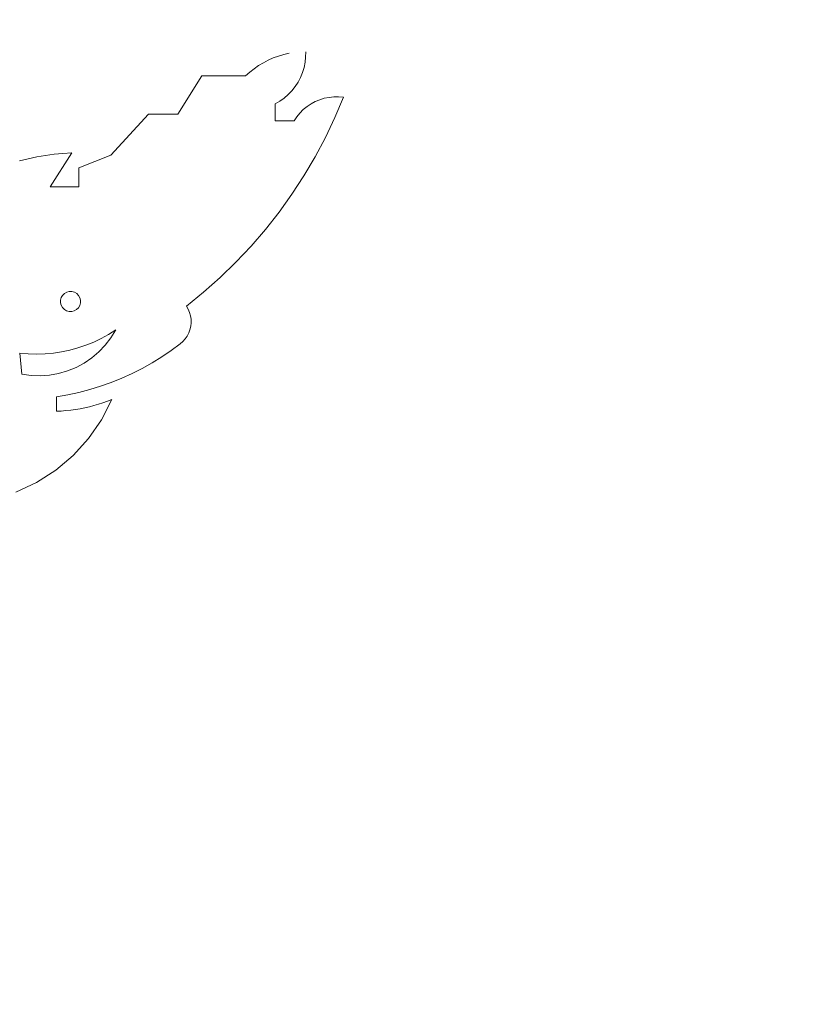
# Model space of a CAD drawing. Units: millimetres. Extents: x 7894 to 8038, y 6851 to 6951.
# Tile 31 of 49: x 7960.68 to 7962.874, y 6925.713 to 6928.453. Entities that reach past the tile are written whole.
import ezdxf

# ---------------------------------------------------------------- set-up
doc = ezdxf.new("R2010")
doc.units = ezdxf.units.MM
doc.layers.add('A-ANNO-DIMS', color=2, linetype='Continuous', lineweight=18)
doc.layers.add('A-FURN-ACCS', color=8, linetype='Continuous', lineweight=13)
doc.styles.get("Standard").update_dxf_attribs({"font": 'arial.ttf'})
doc.dimstyles.new('ISO-25', dxfattribs={"dimtxt": 1, "dimasz": 1, "dimexe": 1.25, "dimexo": 0.625, "dimtad": 1, "dimdec": 0, "dimlunit": 4, "dimtxsty": 'Standard', "dimcen": 2.5, "dimclrt": 1, "dimadec": 0, "dimazin": 0, "dimtfac": 1, "dimtdec": 0, "dimtmove": 0, "dimatfit": 3, "dimfxl": 1, "dimarcsym": 0})

# ---------------------------------------------------------------- blocks, each defined once
blk = doc.blocks.new('DISPLAY-LEAF-FINIAL-Z2_152')
for p, q in [((2.565, 3.5085, 2.1518), (2.5649, 3.4937, 2.1518)), ((2.4472, 3.4779, 2.1518), (2.4609, 3.4849, 2.1518)), ((2.4609, 3.4849, 2.1518), (2.4749, 3.4911, 2.1518)), ((2.4749, 3.4911, 2.1518), (2.4894, 3.4964, 2.1518)), ((2.4894, 3.4964, 2.1518), (2.5041, 3.5007, 2.1518)), ((2.5041, 3.5007, 2.1518), (2.5191, 3.5041, 2.1518)), ((2.5649, 3.4937, 2.1518), (2.5634, 3.479, 2.1518)), ((2.4094, 3.4516, 2.1518), (2.4214, 3.4612, 2.1518)), ((2.4214, 3.4612, 2.1518), (2.4341, 3.4699, 2.1518)), ((2.4341, 3.4699, 2.1518), (2.4472, 3.4779, 2.1518)), ((2.5605, 3.4646, 2.1518), (2.5562, 3.4504, 2.1518)), ((2.5634, 3.479, 2.1518), (2.5605, 3.4646, 2.1518)), ((2.2094, 3.3343, 2.1518), (2.2756, 3.4413, 2.1518)), ((2.2756, 3.4413, 2.1518), (2.3979, 3.4413, 2.1518)), ((2.3979, 3.4413, 2.1518), (2.4094, 3.4516, 2.1518)), ((2.5507, 3.4368, 2.1518), (2.5438, 3.4237, 2.1518)), ((2.5562, 3.4504, 2.1518), (2.5507, 3.4368, 2.1518)), ((2.5266, 3.3997, 2.1518), (2.5164, 3.3891, 2.1518)), ((2.5358, 3.4113, 2.1518), (2.5266, 3.3997, 2.1518)), ((2.5438, 3.4237, 2.1518), (2.5358, 3.4113, 2.1518)), ((2.4932, 3.3709, 2.1518), (2.4804, 3.3636, 2.1518)), ((2.5052, 3.3794, 2.1518), (2.4932, 3.3709, 2.1518)), ((2.5164, 3.3891, 2.1518), (2.5052, 3.3794, 2.1518)), ((2.5917, 3.3696, 2.1518), (2.604, 3.3748, 2.1518)), ((2.604, 3.3748, 2.1518), (2.6168, 3.3788, 2.1518)), ((2.6168, 3.3788, 2.1518), (2.63, 3.3815, 2.1518)), ((2.63, 3.3815, 2.1518), (2.6433, 3.3829, 2.1518)), ((2.6433, 3.3829, 2.1518), (2.6567, 3.3831, 2.1518)), ((2.6701, 3.3819, 2.1518), (2.6462, 3.3254, 2.1518)), ((2.6567, 3.3831, 2.1518), (2.6701, 3.3819, 2.1518)), ((2.4804, 3.3636, 2.1518), (2.4804, 3.3164, 2.1518)), ((2.5489, 3.3378, 2.1518), (2.5584, 3.3473, 2.1518)), ((2.5584, 3.3473, 2.1518), (2.5687, 3.3558, 2.1518)), ((2.5687, 3.3558, 2.1518), (2.5799, 3.3633, 2.1518)), ((2.5799, 3.3633, 2.1518), (2.5917, 3.3696, 2.1518)), ((2.0233, 3.2209, 2.1518), (2.1272, 3.3343, 2.1518)), ((2.1272, 3.3343, 2.1518), (2.2094, 3.3343, 2.1518)), ((2.4804, 3.3164, 2.1518), (2.5329, 3.3164, 2.1518)), ((2.5329, 3.3164, 2.1518), (2.5403, 3.3275, 2.1518)), ((2.5403, 3.3275, 2.1518), (2.5489, 3.3378, 2.1518)), ((2.6462, 3.3254, 2.1518), (2.6199, 3.27, 2.1518)), ((2.6199, 3.27, 2.1518), (2.5912, 3.2159, 2.1518)), ((1.7688, 3.2049, 2.1518), (1.7926, 3.2108, 2.1518)), ((1.7926, 3.2108, 2.1518), (1.8166, 3.2158, 2.1518)), ((1.8166, 3.2158, 2.1518), (1.8408, 3.2199, 2.1518)), ((1.8408, 3.2199, 2.1518), (1.8651, 3.2232, 2.1518)), ((1.9139, 3.2271, 2.1518), (1.8536, 3.1329, 2.1518)), ((1.8651, 3.2232, 2.1518), (1.8895, 3.2256, 2.1518)), ((1.8895, 3.2256, 2.1518), (1.9139, 3.2271, 2.1518)), ((1.934, 3.1854, 2.1518), (2.0233, 3.2209, 2.1518)), ((2.5912, 3.2159, 2.1518), (2.56, 3.1631, 2.1518)), ((1.934, 3.1329, 2.1518), (1.934, 3.1854, 2.1518)), ((2.56, 3.1631, 2.1518), (2.5265, 3.1117, 2.1518)), ((1.8536, 3.1329, 2.1518), (1.934, 3.1329, 2.1518)), ((2.5265, 3.1117, 2.1518), (2.4908, 3.0619, 2.1518)), ((2.4908, 3.0619, 2.1518), (2.4529, 3.0137, 2.1518)), ((2.4529, 3.0137, 2.1518), (2.4129, 2.9672, 2.1518)), ((2.4129, 2.9672, 2.1518), (2.3708, 2.9226, 2.1518)), ((2.3708, 2.9226, 2.1518), (2.3268, 2.8799, 2.1518)), ((2.3268, 2.8799, 2.1518), (2.2809, 2.8392, 2.1518)), ((1.8829, 2.8172, 2.1518), (1.8849, 2.8243, 2.1518)), ((1.8849, 2.8243, 2.1518), (1.8885, 2.8306, 2.1518)), ((1.8885, 2.8306, 2.1518), (1.8937, 2.8357, 2.1518)), ((1.8937, 2.8357, 2.1518), (1.9001, 2.8393, 2.1518)), ((1.9001, 2.8393, 2.1518), (1.9071, 2.8412, 2.1518)), ((1.9071, 2.8412, 2.1518), (1.9144, 2.8411, 2.1518)), ((1.9144, 2.8411, 2.1518), (1.9215, 2.8392, 2.1518)), ((1.9215, 2.8392, 2.1518), (1.9278, 2.8355, 2.1518)), ((1.9278, 2.8355, 2.1518), (1.9329, 2.8304, 2.1518)), ((1.9329, 2.8304, 2.1518), (1.9365, 2.824, 2.1518)), ((1.9365, 2.824, 2.1518), (1.9384, 2.817, 2.1518)), ((2.2809, 2.8392, 2.1518), (2.2333, 2.8006, 2.1518)), ((1.8829, 2.8099, 2.1518), (1.8829, 2.8172, 2.1518)), ((1.8847, 2.8029, 2.1518), (1.8829, 2.8099, 2.1518)), ((1.8884, 2.7965, 2.1518), (1.8847, 2.8029, 2.1518)), ((1.8935, 2.7913, 2.1518), (1.8884, 2.7965, 2.1518)), ((1.9327, 2.7963, 2.1518), (1.9275, 2.7912, 2.1518)), ((1.9364, 2.8026, 2.1518), (1.9327, 2.7963, 2.1518)), ((1.9383, 2.8097, 2.1518), (1.9364, 2.8026, 2.1518)), ((1.9384, 2.817, 2.1518), (1.9383, 2.8097, 2.1518)), ((2.2333, 2.8006, 2.1518), (2.2382, 2.7921, 2.1518)), ((1.8998, 2.7877, 2.1518), (1.8935, 2.7913, 2.1518)), ((1.9068, 2.7857, 2.1518), (1.8998, 2.7877, 2.1518)), ((1.9141, 2.7857, 2.1518), (1.9068, 2.7857, 2.1518)), ((1.9212, 2.7876, 2.1518), (1.9141, 2.7857, 2.1518)), ((1.9275, 2.7912, 2.1518), (1.9212, 2.7876, 2.1518)), ((2.2382, 2.7921, 2.1518), (2.242, 2.7831, 2.1518)), ((2.242, 2.7831, 2.1518), (2.2446, 2.7737, 2.1518)), ((2.2446, 2.7737, 2.1518), (2.246, 2.7641, 2.1518)), ((2.2452, 2.7446, 2.1518), (2.243, 2.7351, 2.1518)), ((2.2462, 2.7543, 2.1518), (2.2452, 2.7446, 2.1518)), ((2.246, 2.7641, 2.1518), (2.2462, 2.7543, 2.1518)), ((2.0167, 2.7218, 2.1518), (1.9962, 2.7106, 2.1518)), ((2.023, 2.7124, 2.1518), (2.0073, 2.692, 2.1518)), ((2.0364, 2.7343, 2.1518), (2.0167, 2.7218, 2.1518)), ((2.0364, 2.7343, 2.1518), (2.023, 2.7124, 2.1518)), ((2.2352, 2.7172, 2.1518), (2.2296, 2.7092, 2.1518)), ((2.2396, 2.7259, 2.1518), (2.2352, 2.7172, 2.1518)), ((2.243, 2.7351, 2.1518), (2.2396, 2.7259, 2.1518)), ((1.9535, 2.6918, 2.1518), (1.9314, 2.6843, 2.1518)), ((1.9751, 2.7005, 2.1518), (1.9535, 2.6918, 2.1518)), ((1.9962, 2.7106, 2.1518), (1.9751, 2.7005, 2.1518)), ((2.0073, 2.692, 2.1518), (1.9895, 2.6734, 2.1518)), ((2.2158, 2.6954, 2.1518), (2.1904, 2.6768, 2.1518)), ((2.2231, 2.7019, 2.1518), (2.2158, 2.6954, 2.1518)), ((2.2296, 2.7092, 2.1518), (2.2231, 2.7019, 2.1518)), ((1.793, 2.6675, 2.1518), (1.7698, 2.6695, 2.1518)), ((1.7698, 2.6695, 2.1518), (1.7755, 2.6114, 2.1518)), ((1.8164, 2.6669, 2.1518), (1.793, 2.6675, 2.1518)), ((1.8397, 2.6677, 2.1518), (1.8164, 2.6669, 2.1518)), ((1.8629, 2.6698, 2.1518), (1.8397, 2.6677, 2.1518)), ((1.886, 2.6733, 2.1518), (1.8629, 2.6698, 2.1518)), ((1.9089, 2.6781, 2.1518), (1.886, 2.6733, 2.1518)), ((1.9314, 2.6843, 2.1518), (1.9089, 2.6781, 2.1518)), ((1.9895, 2.6734, 2.1518), (1.9699, 2.6568, 2.1518)), ((2.1643, 2.6592, 2.1518), (2.1374, 2.6427, 2.1518)), ((2.1904, 2.6768, 2.1518), (2.1643, 2.6592, 2.1518)), ((1.9261, 2.6302, 2.1518), (1.9023, 2.6205, 2.1518)), ((1.9487, 2.6423, 2.1518), (1.9261, 2.6302, 2.1518)), ((1.9699, 2.6568, 2.1518), (1.9487, 2.6423, 2.1518)), ((2.1374, 2.6427, 2.1518), (2.1099, 2.6273, 2.1518)), ((1.8009, 2.6079, 2.1518), (1.7755, 2.6114, 2.1518)), ((1.8266, 2.607, 2.1518), (1.8009, 2.6079, 2.1518)), ((1.8523, 2.6088, 2.1518), (1.8266, 2.607, 2.1518)), ((1.8776, 2.6133, 2.1518), (1.8523, 2.6088, 2.1518)), ((1.9023, 2.6205, 2.1518), (1.8776, 2.6133, 2.1518)), ((2.0818, 2.6132, 2.1518), (2.0531, 2.6002, 2.1518)), ((2.1099, 2.6273, 2.1518), (2.0818, 2.6132, 2.1518)), ((1.9942, 2.5779, 2.1518), (1.9641, 2.5686, 2.1518)), ((2.0239, 2.5884, 2.1518), (1.9942, 2.5779, 2.1518)), ((2.0531, 2.6002, 2.1518), (2.0239, 2.5884, 2.1518)), ((1.9029, 2.5539, 2.1518), (1.8718, 2.5484, 2.1518)), ((1.8718, 2.5484, 2.1518), (1.8718, 2.5082, 2.1518)), ((1.9336, 2.5606, 2.1518), (1.9029, 2.5539, 2.1518)), ((1.9641, 2.5686, 2.1518), (1.9336, 2.5606, 2.1518)), ((1.9502, 2.5177, 2.1518), (1.9631, 2.5206, 2.1518)), ((1.9631, 2.5206, 2.1518), (1.9758, 2.5239, 2.1518)), ((1.9758, 2.5239, 2.1518), (1.9885, 2.5276, 2.1518)), ((1.9885, 2.5276, 2.1518), (2.001, 2.5317, 2.1518)), ((2.0257, 2.5409, 2.1518), (1.9968, 2.4843, 2.1518)), ((2.001, 2.5317, 2.1518), (2.0134, 2.5361, 2.1518)), ((2.0134, 2.5361, 2.1518), (2.0257, 2.5409, 2.1518)), ((1.8718, 2.5082, 2.1518), (1.885, 2.5088, 2.1518)), ((1.885, 2.5088, 2.1518), (1.8981, 2.5098, 2.1518)), ((1.8981, 2.5098, 2.1518), (1.9112, 2.5112, 2.1518)), ((1.9112, 2.5112, 2.1518), (1.9243, 2.513, 2.1518)), ((1.9243, 2.513, 2.1518), (1.9373, 2.5152, 2.1518)), ((1.9373, 2.5152, 2.1518), (1.9502, 2.5177, 2.1518)), ((1.9968, 2.4843, 2.1518), (1.9607, 2.4321, 2.1518)), ((1.9607, 2.4321, 2.1518), (1.918, 2.3851, 2.1518)), ((1.918, 2.3851, 2.1518), (1.8695, 2.3441, 2.1518)), ((1.8695, 2.3441, 2.1518), (1.8161, 2.3099, 2.1518)), ((1.8161, 2.3099, 2.1518), (1.7585, 2.283, 2.1518))]:
    blk.add_line(p, q)
blk = doc.blocks.new('*D23')
at = {"layer": 'A-ANNO-DIMS', "color": 0, "lineweight": -2, "transparency": 16777216}
for p, q in [((7940.0888, 6907.098), (7940.0888, 6947.7928)), ((7971.9356, 6928.989), (7971.9356, 6947.7928)), ((7941.0888, 6946.5428), (7970.9356, 6946.5428))]:
    blk.add_line(p, q, dxfattribs=at)
at = {"layer": 'A-ANNO-DIMS', "color": 0, "transparency": 16777216}
for points in [[(7941.0888, 6946.7095), (7941.0888, 6946.3762), (7940.0888, 6946.5428)], [(7970.9356, 6946.7095), (7970.9356, 6946.3762), (7971.9356, 6946.5428)]]:
    blk.add_solid(points, dxfattribs=at)
at = {"layer": 'Defpoints', "color": 0, "transparency": 16777216}
for p in [(7971.9356, 6946.5428), (7971.9356, 6928.364), (7940.0888, 6906.473)]:
    blk.add_point(p, dxfattribs=at)
at = {"layer": 'A-ANNO-DIMS', "color": 1, "transparency": 16777216, "insert": (7956.0122, 6947.6784), "char_height": 1, "attachment_point": 5}
blk.add_mtext('2\'-8"', dxfattribs=at)
blk = doc.blocks.new('*D28')
at = {"layer": 'A-ANNO-DIMS', "color": 0, "lineweight": -2, "transparency": 16777216}
for p, q in [((7960.8854, 6936.8804), (7975.2272, 6936.8804)), ((7973.9772, 6935.8804), (7973.9772, 6923.6283)), ((7971.8421, 6922.6283), (7975.2272, 6922.6283))]:
    blk.add_line(p, q, dxfattribs=at)
at = {"layer": 'A-ANNO-DIMS', "color": 0, "transparency": 16777216}
for points in [[(7973.8105, 6935.8804), (7974.1439, 6935.8804), (7973.9772, 6936.8804)], [(7973.8105, 6923.6283), (7974.1439, 6923.6283), (7973.9772, 6922.6283)]]:
    blk.add_solid(points, dxfattribs=at)
at = {"layer": 'Defpoints', "color": 0, "transparency": 16777216}
for p in [(7960.2604, 6936.8804), (7971.2171, 6922.6283), (7973.9772, 6922.6283)]:
    blk.add_point(p, dxfattribs=at)
at = {"layer": 'A-ANNO-DIMS', "color": 1, "transparency": 16777216, "insert": (7972.8351, 6929.7543), "char_height": 1, "attachment_point": 5, "rotation": 90}
blk.add_mtext('1\'-2 1/2"', dxfattribs=at)
blk = doc.blocks.new('*D31')
at = {"layer": 'A-ANNO-DIMS', "color": 0, "lineweight": -2, "transparency": 16777216}
for p, q in [((7973.9772, 6921.7198), (7973.9772, 6926.628)), ((7949.8107, 6920.7198), (7975.2272, 6920.7198)), ((7973.9772, 6918.7198), (7973.9772, 6920.7198)), ((7950.9654, 6918.7198), (7975.2272, 6918.7198)), ((7973.9772, 6917.7198), (7973.9772, 6916.7198))]:
    blk.add_line(p, q, dxfattribs=at)
at = {"layer": 'A-ANNO-DIMS', "color": 0, "transparency": 16777216}
for points in [[(7973.8105, 6921.7198), (7974.1439, 6921.7198), (7973.9772, 6920.7198)], [(7973.8105, 6917.7198), (7974.1439, 6917.7198), (7973.9772, 6918.7198)]]:
    blk.add_solid(points, dxfattribs=at)
at = {"layer": 'Defpoints', "color": 0, "transparency": 16777216}
for p in [(7949.1857, 6920.7198), (7973.9772, 6920.7198), (7950.3404, 6918.7198)]:
    blk.add_point(p, dxfattribs=at)
at = {"layer": 'A-ANNO-DIMS', "color": 1, "transparency": 16777216, "insert": (7972.8416, 6924.6739), "char_height": 1, "attachment_point": 5, "rotation": 90}
blk.add_mtext('0\'-2"', dxfattribs=at)

msp = doc.modelspace()

# ---------------------------------------------------------------- block references
at = {"layer": 'A-FURN-ACCS'}
msp.add_blockref('DISPLAY-LEAF-FINIAL-Z2_152', (7958.9107, 6924.8555), dxfattribs=at)

# ---------------------------------------------------------------- dimensions: what is measured, and where the dimension line sits
at = {"layer": 'A-ANNO-DIMS'}
dim = msp.add_linear_dim(base=(7971.9356, 6946.5428), p1=(7940.0888, 6906.473), p2=(7971.9356, 6928.364), dimstyle='ISO-25', override={"dimdec": 1, "dimlfac": 1, "dimrnd": 0, "dimzin": 1, "dimdsep": 46, "dimlunit": 4, "dimfrac": 2}, dxfattribs=at)
dim.commit()
dim.dimension.update_dxf_attribs({"geometry": '*D23', "text_midpoint": (7956.0122, 6947.6784)})
for base, p1, p2, picture, middle in [((7973.9772, 6922.6283), (7960.2604, 6936.8804), (7971.2171, 6922.6283), '*D28', (7972.8351, 6929.7543)), ((7973.9772, 6920.7198), (7950.3404, 6918.7198), (7949.1857, 6920.7198), '*D31', (7972.8416, 6924.6739))]:
    dim = msp.add_linear_dim(base=base, p1=p1, p2=p2, angle=90, dimstyle='ISO-25', override={"dimdec": 1, "dimlfac": 1, "dimrnd": 0, "dimzin": 1, "dimdsep": 46, "dimlunit": 4, "dimfrac": 2}, dxfattribs=at)
    dim.commit()
    dim.dimension.update_dxf_attribs({"geometry": picture, "text_midpoint": middle})

doc.saveas('drawing.dxf')
